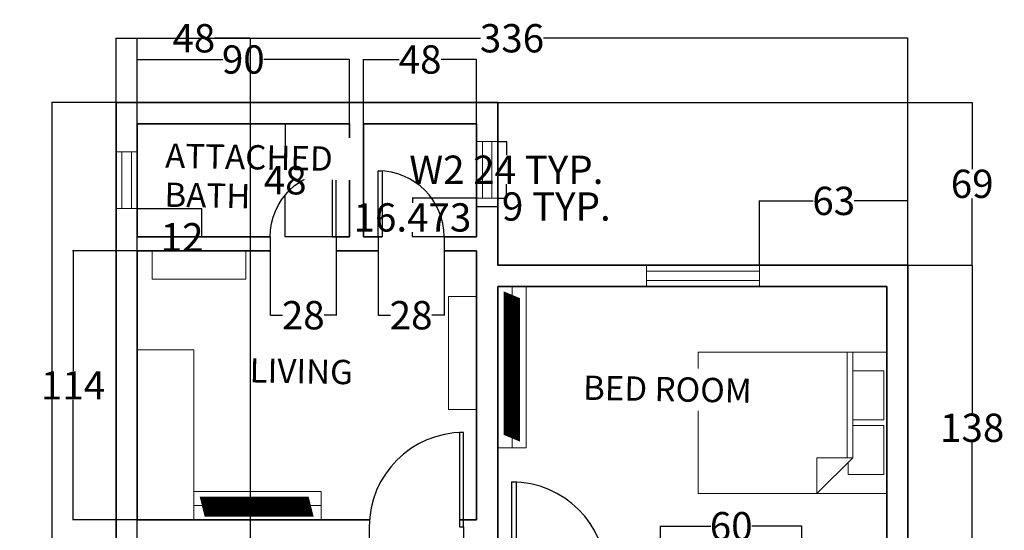
# Model space of a CAD drawing. Units: inches. Extents: x 424 to 1593, y 6 to 578.
# Tile 4 of 4: x 1175 to 1593, y 361 to 578. Entities that reach past the tile are written whole.
import ezdxf

# ---------------------------------------------------------------- set-up
doc = ezdxf.new("R2010")
doc.units = ezdxf.units.IN
doc.header["$MEASUREMENT"] = 0
for name, color, linetype, lineweight in [('A-ANNO-DIMS', 2, 'Continuous', 18), ('A-AREA-IDEN', 7, 'Continuous', 18), ('A-DOOR', 3, 'Continuous', 25), ('A-FLOR-CASE', 9, 'Continuous', 18), ('A-FLOR-CASE-PATT', 252, 'Continuous', 13), ('A-FURN', 8, 'Continuous', 18), ('A-GLAZ', 4, 'Continuous', 18), ('A-WALL', 7, 'Continuous', 35)]:
    doc.layers.add(name, color=color, linetype=linetype, lineweight=lineweight)
doc.styles.get("Standard").update_dxf_attribs({"font": 'arial.ttf'})
doc.dimstyles.get("Standard").update_dxf_attribs({"dimtxt": 12, "dimasz": 0.18, "dimexe": 0.18, "dimexo": 0.0625, "dimgap": 0.09, "dimtad": 0, "dimtih": 1, "dimtoh": 1, "dimdec": 0, "dimzin": 0, "dimdsep": 46, "dimlunit": 3, "dimtxsty": 'Standard', "dimcen": 0.09, "dimadec": 0, "dimazin": 0, "dimtfac": 1, "dimtdec": 0, "dimtofl": 0, "dimtmove": 0, "dimatfit": 3, "dimfxl": 1, "dimtolj": 1, "dimtzin": 0, "dimarcsym": 0})

# ---------------------------------------------------------------- blocks, each defined once
blk = doc.blocks.new('*U3')
for p, q in [((0, 0), (0, -6)), ((-40, 0), (-40, -6))]:
    blk.add_line(p, q)
blk.add_lwpolyline([(0, 0), (0, 40), (-1.75, 40), (-1.75, 0)], close=True)
blk.add_arc((0, 0), 40, 90, 180)
blk = doc.blocks.new('*U6')
for p, q in [((0, 0), (0, -6)), ((40, 0), (40, -6))]:
    blk.add_line(p, q)
blk.add_lwpolyline([(0, 0), (0, 40), (1.75, 40), (1.75, 0)], close=True)
blk.add_arc((0, 0), 40, 0, 90)
blk = doc.blocks.new('*U7')
for p, q in [((0, 0), (0, -6)), ((28, 0), (28, -6))]:
    blk.add_line(p, q)
blk.add_lwpolyline([(0, 0), (0, 28), (1.75, 28), (1.75, 0)], close=True)
blk.add_arc((0, 0), 28, 0, 90)
blk = doc.blocks.new('Bed - Queen')
for p, q in [((0, -80.00003), (0, 0)), ((0, 0), (59.99999, 0)), ((59.99999, 0), (59.99999, -80.00003)), ((7.99999, -1.2), (28.79998, -1.2)), ((7.99999, -14.4), (7.99999, -1.2)), ((28.79998, -1.2), (28.79998, -14.4)), ((31.19999, -1.2), (51.99999, -1.2)), ((31.19999, -14.4), (31.19999, -1.2)), ((51.99999, -1.2), (51.99999, -16.4)), ((0, -14.4), (44.8, -14.4)), ((59.99999, -29.6), (44.8, -14.4)), ((44.8, -14.4), (44.8, -29.6)), ((51.99999, -16.4), (46.79936, -16.4)), ((44.8, -16.8), (0, -16.8)), ((44.8, -29.6), (59.99999, -29.6)), ((59.99999, -80.00003), (0, -80.00003))]:
    blk.add_line(p, q)
blk = doc.blocks.new('WIN-48IN')
for p, q in [((2.5, 48), (2.5, 0)), ((6.5, 48), (6.5, 0))]:
    blk.add_line(p, q)
blk.add_lwpolyline([(0, 48), (9, 48), (9, 0), (0, 0)], close=True)
blk = doc.blocks.new('WIN-24IN')
for p, q in [((2.5, 0), (2.5, 24)), ((6.5, 0), (6.5, 24))]:
    blk.add_line(p, q)
blk.add_lwpolyline([(9, 0), (0, 0), (0, 24), (9, 24)], close=True)
blk = doc.blocks.new('CASEWORK-48X12')
blk.add_lwpolyline([(12, 48), (0, 48), (0, 0), (12, 0)], close=True)
blk = doc.blocks.new('*D14')
at = {"layer": 'A-ANNO-DIMS', "color": 0, "lineweight": -2, "transparency": 16777216}
for p, q in [((1377.79, 526), (1381.51, 526)), ((1381.33, 525.82), (1381.33, 520.12)), ((1381.33, 502.18), (1381.33, 507.88)), ((1377.79, 502), (1381.51, 502))]:
    blk.add_line(p, q, dxfattribs=at)
at = {"layer": 'A-ANNO-DIMS', "color": 0, "transparency": 16777216}
for points in [[(1381.3, 525.82), (1381.36, 525.82), (1381.33, 526)], [(1381.3, 502.18), (1381.36, 502.18), (1381.33, 502)]]:
    blk.add_solid(points, dxfattribs=at)
at = {"layer": 'Defpoints', "color": 0, "transparency": 16777216}
for p in [(1377.73, 526), (1381.33, 526), (1377.73, 502)]:
    blk.add_point(p, dxfattribs=at)
at = {"layer": 'A-ANNO-DIMS', "color": 0, "transparency": 16777216, "insert": (1381.33, 514), "char_height": 12, "attachment_point": 5}
blk.add_mtext('\\A1;W2 24 TYP.', dxfattribs=at)
blk = doc.blocks.new('*D15')
at = {"layer": 'A-ANNO-DIMS', "color": 0, "lineweight": -2, "transparency": 16777216}
for p, q in [((1368.73, 501.94), (1368.73, 498.22)), ((1377.73, 501.94), (1377.73, 498.22)), ((1368.91, 498.4), (1377.55, 498.4)), ((1377.73, 498.4), (1377.91, 498.4))]:
    blk.add_line(p, q, dxfattribs=at)
at = {"layer": 'A-ANNO-DIMS', "color": 0, "transparency": 16777216}
for points in [[(1368.91, 498.43), (1368.91, 498.37), (1368.73, 498.4)], [(1377.55, 498.43), (1377.55, 498.37), (1377.73, 498.4)]]:
    blk.add_solid(points, dxfattribs=at)
at = {"layer": 'Defpoints', "color": 0, "transparency": 16777216}
for p in [(1368.73, 502), (1377.73, 502), (1377.73, 498.4)]:
    blk.add_point(p, dxfattribs=at)
at = {"layer": 'A-ANNO-DIMS', "color": 0, "transparency": 16777216, "insert": (1402.54, 498.4), "char_height": 12, "attachment_point": 5}
blk.add_mtext('\\A1;9 TYP.', dxfattribs=at)
blk = doc.blocks.new('*D48')
at = {"layer": 'A-ANNO-DIMS', "color": 0, "lineweight": -2, "transparency": 16777216}
for p, q in [((1215.73, 542.59), (1215.73, 569.96)), ((1215.91, 569.78), (1370.39, 569.78)), ((1551.55, 569.78), (1397.07, 569.78)), ((1551.73, 473.59), (1551.73, 569.96))]:
    blk.add_line(p, q, dxfattribs=at)
at = {"layer": 'A-ANNO-DIMS', "color": 0, "transparency": 16777216}
for points in [[(1215.91, 569.81), (1215.91, 569.75), (1215.73, 569.78)], [(1551.55, 569.81), (1551.55, 569.75), (1551.73, 569.78)]]:
    blk.add_solid(points, dxfattribs=at)
at = {"layer": 'Defpoints', "color": 0, "transparency": 16777216}
for p in [(1551.73, 569.78), (1215.73, 542.53), (1551.73, 473.53)]:
    blk.add_point(p, dxfattribs=at)
at = {"layer": 'A-ANNO-DIMS', "color": 0, "transparency": 16777216, "insert": (1383.73, 569.78), "char_height": 12, "attachment_point": 5}
blk.add_mtext('\\A1;336', dxfattribs=at)
blk = doc.blocks.new('*D49')
at = {"layer": 'A-ANNO-DIMS', "color": 0, "lineweight": -2, "transparency": 16777216}
for p, q in [((1215.66, 542.53), (1188.3, 542.53)), ((1188.48, 542.35), (1188.48, 302.75)), ((1188.48, 50.71), (1188.48, 290.31)), ((1215.66, 50.53), (1188.3, 50.53))]:
    blk.add_line(p, q, dxfattribs=at)
at = {"layer": 'A-ANNO-DIMS', "color": 0, "transparency": 16777216}
for points in [[(1188.45, 542.35), (1188.51, 542.35), (1188.48, 542.53)], [(1188.45, 50.71), (1188.51, 50.71), (1188.48, 50.53)]]:
    blk.add_solid(points, dxfattribs=at)
at = {"layer": 'Defpoints', "color": 0, "transparency": 16777216}
for p in [(1188.48, 542.53), (1215.73, 542.53), (1215.73, 50.53)]:
    blk.add_point(p, dxfattribs=at)
at = {"layer": 'A-ANNO-DIMS', "color": 0, "transparency": 16777216, "insert": (1188.48, 296.53), "char_height": 12, "attachment_point": 5}
blk.add_mtext('\\A1;492', dxfattribs=at)
blk = doc.blocks.new('*D53')
at = {"layer": 'A-ANNO-DIMS', "color": 0, "lineweight": -2, "transparency": 16777216}
for p, q in [((1224.66, 479.53), (1197.3, 479.53)), ((1197.48, 479.35), (1197.48, 428.64)), ((1197.48, 365.71), (1197.48, 416.42)), ((1224.66, 365.53), (1197.3, 365.53))]:
    blk.add_line(p, q, dxfattribs=at)
at = {"layer": 'A-ANNO-DIMS', "color": 0, "transparency": 16777216}
for points in [[(1197.45, 479.35), (1197.51, 479.35), (1197.48, 479.53)], [(1197.45, 365.71), (1197.51, 365.71), (1197.48, 365.53)]]:
    blk.add_solid(points, dxfattribs=at)
at = {"layer": 'Defpoints', "color": 0, "transparency": 16777216}
for p in [(1197.48, 479.53), (1224.73, 479.53), (1224.73, 365.53)]:
    blk.add_point(p, dxfattribs=at)
at = {"layer": 'A-ANNO-DIMS', "color": 0, "transparency": 16777216, "insert": (1197.48, 422.53), "char_height": 12, "attachment_point": 5}
blk.add_mtext('\\A1;114', dxfattribs=at)
blk = doc.blocks.new('*D54')
at = {"layer": 'A-ANNO-DIMS', "color": 0, "lineweight": -2, "transparency": 16777216}
for p, q in [((1314.66, 533.53), (1287.3, 533.53)), ((1287.48, 533.35), (1287.48, 515.75)), ((1287.48, 485.71), (1287.48, 503.31)), ((1314.66, 485.53), (1287.3, 485.53))]:
    blk.add_line(p, q, dxfattribs=at)
at = {"layer": 'A-ANNO-DIMS', "color": 0, "transparency": 16777216}
for points in [[(1287.45, 533.35), (1287.51, 533.35), (1287.48, 533.53)], [(1287.45, 485.71), (1287.51, 485.71), (1287.48, 485.53)]]:
    blk.add_solid(points, dxfattribs=at)
at = {"layer": 'Defpoints', "color": 0, "transparency": 16777216}
for p in [(1287.48, 533.53), (1314.73, 533.53), (1314.73, 485.53)]:
    blk.add_point(p, dxfattribs=at)
at = {"layer": 'A-ANNO-DIMS', "color": 0, "transparency": 16777216, "insert": (1287.48, 509.53), "char_height": 12, "attachment_point": 5}
blk.add_mtext('\\A1;48', dxfattribs=at)
blk = doc.blocks.new('*D58')
at = {"layer": 'A-ANNO-DIMS', "color": 0, "lineweight": -2, "transparency": 16777216}
for p, q in [((1551.79, 473.53), (1579.16, 473.53)), ((1578.98, 473.35), (1578.98, 410.75)), ((1578.98, 335.71), (1578.98, 398.31)), ((1542.79, 335.53), (1579.16, 335.53))]:
    blk.add_line(p, q, dxfattribs=at)
at = {"layer": 'A-ANNO-DIMS', "color": 0, "transparency": 16777216}
for points in [[(1578.95, 473.35), (1579.01, 473.35), (1578.98, 473.53)], [(1578.95, 335.71), (1579.01, 335.71), (1578.98, 335.53)]]:
    blk.add_solid(points, dxfattribs=at)
at = {"layer": 'Defpoints', "color": 0, "transparency": 16777216}
for p in [(1551.73, 473.53), (1578.98, 473.53), (1542.73, 335.53)]:
    blk.add_point(p, dxfattribs=at)
at = {"layer": 'A-ANNO-DIMS', "color": 0, "transparency": 16777216, "insert": (1578.98, 404.53), "char_height": 12, "attachment_point": 5}
blk.add_mtext('\\A1;138', dxfattribs=at)
blk = doc.blocks.new('*D59')
at = {"layer": 'A-ANNO-DIMS', "color": 0, "lineweight": -2, "transparency": 16777216}
for p, q in [((1377.79, 542.53), (1579.16, 542.53)), ((1578.98, 542.35), (1578.98, 514.25)), ((1578.98, 473.71), (1578.98, 501.81)), ((1551.79, 473.53), (1579.16, 473.53))]:
    blk.add_line(p, q, dxfattribs=at)
at = {"layer": 'A-ANNO-DIMS', "color": 0, "transparency": 16777216}
for points in [[(1578.95, 542.35), (1579.01, 542.35), (1578.98, 542.53)], [(1578.95, 473.71), (1579.01, 473.71), (1578.98, 473.53)]]:
    blk.add_solid(points, dxfattribs=at)
at = {"layer": 'Defpoints', "color": 0, "transparency": 16777216}
for p in [(1377.73, 542.53), (1578.98, 542.53), (1551.73, 473.53)]:
    blk.add_point(p, dxfattribs=at)
at = {"layer": 'A-ANNO-DIMS', "color": 0, "transparency": 16777216, "insert": (1578.98, 508.03), "char_height": 12, "attachment_point": 5}
blk.add_mtext('\\A1;69', dxfattribs=at)
blk = doc.blocks.new('*D60')
at = {"layer": 'A-ANNO-DIMS', "color": 0, "lineweight": -2, "transparency": 16777216}
for p, q in [((1224.73, 533.59), (1224.73, 560.96)), ((1224.91, 560.78), (1261.06, 560.78)), ((1314.55, 560.78), (1278.39, 560.78)), ((1314.73, 533.59), (1314.73, 560.96))]:
    blk.add_line(p, q, dxfattribs=at)
at = {"layer": 'A-ANNO-DIMS', "color": 0, "transparency": 16777216}
for points in [[(1224.91, 560.81), (1224.91, 560.75), (1224.73, 560.78)], [(1314.55, 560.81), (1314.55, 560.75), (1314.73, 560.78)]]:
    blk.add_solid(points, dxfattribs=at)
at = {"layer": 'Defpoints', "color": 0, "transparency": 16777216}
for p in [(1314.73, 560.78), (1224.73, 533.53), (1314.73, 533.53)]:
    blk.add_point(p, dxfattribs=at)
at = {"layer": 'A-ANNO-DIMS', "color": 0, "transparency": 16777216, "insert": (1269.73, 560.78), "char_height": 12, "attachment_point": 5}
blk.add_mtext('\\A1;90', dxfattribs=at)
blk = doc.blocks.new('*D61')
at = {"layer": 'A-ANNO-DIMS', "color": 0, "lineweight": -2, "transparency": 16777216}
for p, q in [((1320.73, 533.59), (1320.73, 560.96)), ((1320.91, 560.78), (1335.79, 560.78)), ((1368.55, 560.78), (1353.67, 560.78)), ((1368.73, 533.59), (1368.73, 560.96))]:
    blk.add_line(p, q, dxfattribs=at)
at = {"layer": 'A-ANNO-DIMS', "color": 0, "transparency": 16777216}
for points in [[(1320.91, 560.81), (1320.91, 560.75), (1320.73, 560.78)], [(1368.55, 560.81), (1368.55, 560.75), (1368.73, 560.78)]]:
    blk.add_solid(points, dxfattribs=at)
at = {"layer": 'Defpoints', "color": 0, "transparency": 16777216}
for p in [(1368.73, 560.78), (1320.73, 533.53), (1368.73, 533.53)]:
    blk.add_point(p, dxfattribs=at)
at = {"layer": 'A-ANNO-DIMS', "color": 0, "transparency": 16777216, "insert": (1344.73, 560.78), "char_height": 12, "attachment_point": 5}
blk.add_mtext('\\A1;48', dxfattribs=at)
blk = doc.blocks.new('*D63')
at = {"layer": 'A-ANNO-DIMS', "color": 0, "lineweight": -2, "transparency": 16777216}
for p, q in [((1224.73, 59.59), (1224.73, 569.96)), ((1224.91, 569.78), (1239.79, 569.78)), ((1272.55, 569.78), (1257.67, 569.78)), ((1272.73, 59.59), (1272.73, 569.96))]:
    blk.add_line(p, q, dxfattribs=at)
at = {"layer": 'A-ANNO-DIMS', "color": 0, "transparency": 16777216}
for points in [[(1224.91, 569.81), (1224.91, 569.75), (1224.73, 569.78)], [(1272.55, 569.81), (1272.55, 569.75), (1272.73, 569.78)]]:
    blk.add_solid(points, dxfattribs=at)
at = {"layer": 'Defpoints', "color": 0, "transparency": 16777216}
for p in [(1272.73, 569.78), (1224.73, 59.53), (1272.73, 59.53)]:
    blk.add_point(p, dxfattribs=at)
at = {"layer": 'A-ANNO-DIMS', "color": 0, "transparency": 16777216, "insert": (1248.73, 569.78), "char_height": 12, "attachment_point": 5}
blk.add_mtext('\\A1;48', dxfattribs=at)
blk = doc.blocks.new('*D64')
at = {"layer": 'A-ANNO-DIMS', "color": 0, "lineweight": -2, "transparency": 16777216}
for p, q in [((1488.73, 473.59), (1488.73, 500.96)), ((1488.91, 500.78), (1511.51, 500.78)), ((1551.55, 500.78), (1528.95, 500.78)), ((1551.73, 473.59), (1551.73, 500.96))]:
    blk.add_line(p, q, dxfattribs=at)
at = {"layer": 'A-ANNO-DIMS', "color": 0, "transparency": 16777216}
for points in [[(1488.91, 500.81), (1488.91, 500.75), (1488.73, 500.78)], [(1551.55, 500.81), (1551.55, 500.75), (1551.73, 500.78)]]:
    blk.add_solid(points, dxfattribs=at)
at = {"layer": 'Defpoints', "color": 0, "transparency": 16777216}
for p in [(1551.73, 500.78), (1488.73, 473.53), (1551.73, 473.53)]:
    blk.add_point(p, dxfattribs=at)
at = {"layer": 'A-ANNO-DIMS', "color": 0, "transparency": 16777216, "insert": (1520.23, 500.78), "char_height": 12, "attachment_point": 5}
blk.add_mtext('\\A1;63', dxfattribs=at)
blk = doc.blocks.new('*D67')
at = {"layer": 'A-ANNO-DIMS', "color": 0, "lineweight": -2, "transparency": 16777216}
for p, q in [((1446.73, 335.59), (1446.73, 362.96)), ((1446.91, 362.78), (1468.03, 362.78)), ((1506.55, 362.78), (1485.42, 362.78)), ((1506.73, 335.59), (1506.73, 362.96))]:
    blk.add_line(p, q, dxfattribs=at)
at = {"layer": 'A-ANNO-DIMS', "color": 0, "transparency": 16777216}
for points in [[(1446.91, 362.81), (1446.91, 362.75), (1446.73, 362.78)], [(1506.55, 362.81), (1506.55, 362.75), (1506.73, 362.78)]]:
    blk.add_solid(points, dxfattribs=at)
at = {"layer": 'Defpoints', "color": 0, "transparency": 16777216}
for p in [(1506.73, 362.78), (1446.73, 335.53), (1506.73, 335.53)]:
    blk.add_point(p, dxfattribs=at)
at = {"layer": 'A-ANNO-DIMS', "color": 0, "transparency": 16777216, "insert": (1476.73, 362.78), "char_height": 12, "attachment_point": 5}
blk.add_mtext('\\A1;60', dxfattribs=at)
blk = doc.blocks.new('*D69')
at = {"layer": 'A-ANNO-DIMS', "color": 0, "lineweight": -2, "transparency": 16777216}
for p, q in [((1224.79, 497.53), (1252.16, 497.53)), ((1251.98, 497.35), (1251.98, 485.71)), ((1224.79, 485.53), (1252.16, 485.53)), ((1251.98, 485.35), (1251.8, 485.35)), ((1251.98, 485.53), (1251.98, 485.35))]:
    blk.add_line(p, q, dxfattribs=at)
at = {"layer": 'A-ANNO-DIMS', "color": 0, "transparency": 16777216}
for points in [[(1251.95, 497.35), (1252.01, 497.35), (1251.98, 497.53)], [(1251.95, 485.71), (1252.01, 485.71), (1251.98, 485.53)]]:
    blk.add_solid(points, dxfattribs=at)
at = {"layer": 'Defpoints', "color": 0, "transparency": 16777216}
for p in [(1224.73, 497.53), (1224.73, 485.53), (1251.98, 485.53)]:
    blk.add_point(p, dxfattribs=at)
at = {"layer": 'A-ANNO-DIMS', "color": 0, "transparency": 16777216, "insert": (1243.74, 485.35), "char_height": 12, "attachment_point": 5}
blk.add_mtext('\\A1;12', dxfattribs=at)
blk = doc.blocks.new('*D70')
at = {"layer": 'A-ANNO-DIMS', "color": 0, "lineweight": -2, "transparency": 16777216}
for p, q in [((1368.66, 502), (1341.3, 502)), ((1341.48, 501.82), (1341.48, 499.99)), ((1368.66, 485.53), (1341.3, 485.53)), ((1341.48, 485.71), (1341.48, 487.55))]:
    blk.add_line(p, q, dxfattribs=at)
at = {"layer": 'A-ANNO-DIMS', "color": 0, "transparency": 16777216}
for points in [[(1341.45, 501.82), (1341.51, 501.82), (1341.48, 502)], [(1341.45, 485.71), (1341.51, 485.71), (1341.48, 485.53)]]:
    blk.add_solid(points, dxfattribs=at)
at = {"layer": 'Defpoints', "color": 0, "transparency": 16777216}
for p in [(1341.48, 502), (1368.73, 502), (1368.73, 485.53)]:
    blk.add_point(p, dxfattribs=at)
at = {"layer": 'A-ANNO-DIMS', "color": 0, "transparency": 16777216, "insert": (1341.48, 493.77), "char_height": 12, "attachment_point": 5}
blk.add_mtext('\\A1;16.473', dxfattribs=at)
blk = doc.blocks.new('*D72')
at = {"layer": 'A-ANNO-DIMS', "color": 0, "lineweight": -2, "transparency": 16777216}
for p, q in [((1281.17, 479.47), (1281.17, 452.1)), ((1309.17, 479.47), (1309.17, 452.1)), ((1281.35, 452.28), (1286.37, 452.28)), ((1308.99, 452.28), (1303.97, 452.28))]:
    blk.add_line(p, q, dxfattribs=at)
at = {"layer": 'A-ANNO-DIMS', "color": 0, "transparency": 16777216}
for points in [[(1281.35, 452.31), (1281.35, 452.25), (1281.17, 452.28)], [(1308.99, 452.31), (1308.99, 452.25), (1309.17, 452.28)]]:
    blk.add_solid(points, dxfattribs=at)
at = {"layer": 'Defpoints', "color": 0, "transparency": 16777216}
for p in [(1281.17, 479.53), (1309.17, 479.53), (1281.17, 452.28)]:
    blk.add_point(p, dxfattribs=at)
at = {"layer": 'A-ANNO-DIMS', "color": 0, "transparency": 16777216, "insert": (1295.17, 452.28), "char_height": 12, "attachment_point": 5}
blk.add_mtext('\\A1;28', dxfattribs=at)
blk = doc.blocks.new('*D73')
at = {"layer": 'A-ANNO-DIMS', "color": 0, "lineweight": -2, "transparency": 16777216}
for p, q in [((1326.92, 479.47), (1326.92, 452.1)), ((1354.92, 479.47), (1354.92, 452.1)), ((1327.1, 452.28), (1332.12, 452.28)), ((1354.74, 452.28), (1349.71, 452.28))]:
    blk.add_line(p, q, dxfattribs=at)
at = {"layer": 'A-ANNO-DIMS', "color": 0, "transparency": 16777216}
for points in [[(1327.1, 452.31), (1327.1, 452.25), (1326.92, 452.28)], [(1354.74, 452.31), (1354.74, 452.25), (1354.92, 452.28)]]:
    blk.add_solid(points, dxfattribs=at)
at = {"layer": 'Defpoints', "color": 0, "transparency": 16777216}
for p in [(1326.92, 479.53), (1354.92, 479.53), (1326.92, 452.28)]:
    blk.add_point(p, dxfattribs=at)
at = {"layer": 'A-ANNO-DIMS', "color": 0, "transparency": 16777216, "insert": (1340.92, 452.28), "char_height": 12, "attachment_point": 5}
blk.add_mtext('\\A1;28', dxfattribs=at)

msp = doc.modelspace()

# ---------------------------------------------------------------- hatches: boundary and pattern name
at = {"layer": 'A-FLOR-CASE-PATT'}
h = msp.add_hatch(dxfattribs=at)
h.set_pattern_fill('ANSI31', color=256, scale=1.178482, angle=112.399, style=0)
h.paths.add_polyline_path([(1380.271, 401.5574), (1387.0743, 398.7254), (1387.0743, 459.5193), (1380.271, 462.3513)])
h = msp.add_hatch(dxfattribs=at)
h.set_pattern_fill('ANSI31', color=256, scale=0.876872, angle=59.407, style=0)
h.paths.add_polyline_path([(1251.353, 375.2477), (1253.4904, 366.927), (1299.4817, 366.927), (1297.3443, 375.2477)])

# ---------------------------------------------------------------- linework, layer by layer
at = {"layer": 'A-FLOR-CASE'}
for p, q in [((1383.7275, 396.0092), (1383.7275, 464.5296)), ((1248.7275, 371.5296), (1302.7275, 371.5296))]:
    msp.add_line(p, q, dxfattribs=at)
for points in [[(1231.0828, 479.5296), (1270.7906, 479.5296), (1270.7906, 467.5296), (1231.0828, 467.5296)], [(1377.7275, 464.5296), (1389.7275, 464.5296), (1389.7275, 396.0092), (1377.7275, 396.0092)], [(1224.7275, 365.5296), (1248.7275, 365.5296), (1248.7275, 437.5296), (1224.7275, 437.5296)], [(1248.7275, 365.5296), (1302.7275, 365.5296), (1302.7275, 377.5296), (1248.7275, 377.5296)]]:
    msp.add_lwpolyline(points, close=True, dxfattribs=at)
at = {"layer": 'A-WALL'}
for p, q in [((1377.7275, 473.5296), (1377.7275, 542.5296)), ((1224.7275, 533.5296), (1314.7275, 533.5296)), ((1224.7275, 485.5296), (1224.7275, 533.5296)), ((1314.7275, 485.5296), (1314.7275, 533.5296)), ((1320.7275, 485.5296), (1320.7275, 533.5296)), ((1320.7275, 533.5296), (1368.7275, 533.5296)), ((1368.7275, 485.5296), (1368.7275, 533.5296)), ((1224.7275, 485.5296), (1281.1668, 485.5296)), ((1307.4168, 485.5296), (1314.7275, 485.5296)), ((1320.7275, 485.5296), (1328.665, 485.5296)), ((1354.915, 485.5296), (1368.7275, 485.5296)), ((1224.7275, 479.5296), (1281.1668, 479.5296)), ((1224.7275, 365.5296), (1224.7275, 479.5296)), ((1309.1668, 479.5296), (1326.915, 479.5296)), ((1326.915, 479.5296), (1320.915, 479.5296)), ((1354.915, 479.5296), (1368.7275, 479.5296)), ((1368.7275, 464.5296), (1368.7275, 479.5296)), ((1377.7275, 473.5296), (1551.7275, 473.5296)), ((1368.7275, 464.5296), (1368.7275, 365.5296)), ((1377.7275, 464.5296), (1542.7275, 464.5296)), ((1377.7275, 464.5296), (1377.7275, 344.5296)), ((1542.7275, 464.5296), (1542.7275, 344.5296)), ((1224.7275, 365.5296), (1323.2714, 365.5296)), ((1361.4088, 365.5296), (1368.7275, 365.5296))]:
    msp.add_line(p, q, dxfattribs=at)
for points in [[(1377.7275, 50.5296), (1215.7275, 50.5296), (1215.7275, 542.5296), (1377.7275, 542.5296)], [(1377.7275, 50.5296), (1215.7275, 50.5296), (1215.7275, 542.5296), (1377.7275, 542.5296)], [(1224.7275, 485.5296), (1224.7275, 533.5296), (1314.7275, 533.5296)], [(1320.7275, 533.5296), (1368.7275, 533.5296)], [(1224.7275, 365.5296), (1224.7275, 479.5296)], [(1551.7275, 473.5296), (1551.7275, 110.5296)], [(1542.7275, 464.5296), (1542.7275, 344.5296)]]:
    msp.add_lwpolyline(points, dxfattribs=at)

# ---------------------------------------------------------------- block references
at = {"layer": 'A-DOOR', "xscale": -1}
msp.add_blockref('*U7', (1309.1668, 485.5296), dxfattribs=at)
at = {"layer": 'A-DOOR'}
for name, p in [('*U7', (1326.915, 485.5296)), ('*U3', (1363.1588, 362.5296)), ('*U6', (1383.7159, 341.5296))]:
    msp.add_blockref(name, p, dxfattribs=at)
at = {"layer": 'A-FLOR-CASE'}
msp.add_blockref('CASEWORK-48X12', (1356.7276, 412.266), dxfattribs=at)
at = {"layer": 'A-FURN', "rotation": 270}
msp.add_blockref('Bed - Queen', (1542.7275, 436.6366), dxfattribs=at)
at = {"layer": 'A-GLAZ'}
for p in [(1368.727, 502.003), (1215.727, 497.5297)]:
    msp.add_blockref('WIN-24IN', p, dxfattribs=at)
at = {"layer": 'A-GLAZ', "rotation": 89.99999999999996}
msp.add_blockref('WIN-48IN', (1488.7276, 464.5297), dxfattribs=at)

# ---------------------------------------------------------------- texts
at = {"layer": 'A-AREA-IDEN'}
for s, p in [('BATH', (1236.1855, 498.3095)), ('LIVING', (1272.3204, 423.7817))]:
    msp.add_text(s, height=10.30671, rotation=358.915866, dxfattribs=at).set_placement(p)

# ---------------------------------------------------------------- dimensions: what is measured, and where the dimension line sits
at = {"layer": 'A-ANNO-DIMS'}
for base, p1, p2, picture, middle in [((1314.7275, 560.7796), (1224.7275, 533.5296), (1314.7275, 533.5296), '*D60', (1269.7275, 560.7796)), ((1368.7275, 560.7796), (1320.7275, 533.5296), (1368.7275, 533.5296), '*D61', (1344.7275, 560.7796)), ((1506.7275, 362.7796), (1446.7275, 335.5296), (1506.7275, 335.5296), '*D67', (1476.7275, 362.7796))]:
    dim = msp.add_linear_dim(base=base, p1=p1, p2=p2, dimstyle='Standard', override={"dimdec": 0, "dimlfac": 1, "dimrnd": 0, "dimzin": 0, "dimdsep": 46, "dimlunit": 2}, dxfattribs=at)
    dim.commit()
    dim.dimension.update_dxf_attribs({"geometry": picture, "text_midpoint": middle})
for base, p1, p2, angle, override, picture, middle in [((1188.4775, 542.5296), (1215.7275, 50.5296), (1215.7275, 542.5296), 90, {"dimdec": 0, "dimlfac": 1, "dimrnd": 0, "dimzin": 0, "dimdsep": 46, "dimlunit": 2}, '*D49', (1188.4775, 296.5296)), ((1578.9775, 542.5296), (1551.7275, 473.5296), (1377.7275, 542.5296), 90, {"dimdec": 0, "dimlfac": 1, "dimrnd": 0, "dimzin": 0, "dimdsep": 46, "dimlunit": 2}, '*D59', (1578.9775, 508.0296)), ((1551.7275, 500.7796), (1488.7275, 473.5296), (1551.7275, 473.5296), 0, {"dimdec": 0, "dimlfac": 1, "dimrnd": 0, "dimzin": 0, "dimdsep": 46, "dimlunit": 2}, '*D64', (1520.2275, 500.7796)), ((1341.4775, 502.0029), (1368.7275, 485.5296), (1368.7275, 502.0029), 90, {"dimdec": 3, "dimlfac": 1, "dimrnd": 0, "dimzin": 0, "dimdsep": 46, "dimlunit": 2}, '*D70', (1341.4775, 493.7663)), ((1251.9775, 485.5296), (1224.7275, 497.5296), (1224.7275, 485.5296), 270, {"dimdec": 0, "dimlfac": 1, "dimrnd": 0, "dimzin": 0, "dimdsep": 46, "dimlunit": 2}, '*D69', (1243.7389, 485.3496)), ((1197.4775, 479.5296), (1224.7275, 365.5296), (1224.7275, 479.5296), 90, {"dimdec": 0, "dimlfac": 1, "dimrnd": 0, "dimzin": 0, "dimdsep": 46, "dimlunit": 2}, '*D53', (1197.4775, 422.5296)), ((1281.1668, 452.2796), (1309.1668, 479.5296), (1281.1668, 479.5296), 180, {"dimdec": 0, "dimlfac": 1, "dimrnd": 0, "dimzin": 0, "dimdsep": 46, "dimlunit": 2}, '*D72', (1295.1668, 452.2796)), ((1326.915, 452.2796), (1354.915, 479.5296), (1326.915, 479.5296), 180, {"dimdec": 0, "dimlfac": 1, "dimrnd": 0, "dimzin": 0, "dimdsep": 46, "dimlunit": 2}, '*D73', (1340.915, 452.2796)), ((1578.9775, 473.5296), (1542.7275, 335.5296), (1551.7275, 473.5296), 90, {"dimdec": 0, "dimlfac": 1, "dimrnd": 0, "dimzin": 0, "dimdsep": 46, "dimlunit": 2}, '*D58', (1578.9775, 404.5296))]:
    dim = msp.add_linear_dim(base=base, p1=p1, p2=p2, angle=angle, dimstyle='Standard', override=override, dxfattribs=at)
    dim.commit()
    dim.dimension.update_dxf_attribs({"geometry": picture, "text_midpoint": middle})
dim = msp.add_linear_dim(base=(1381.3275, 526.0029), p1=(1377.7275, 502.0029), p2=(1377.7275, 526.0029), angle=90, text='W2 <> TYP.', dimstyle='Standard', override={"dimdec": 0, "dimlfac": 1, "dimrnd": 0, "dimzin": 0, "dimdsep": 46, "dimlunit": 2}, dxfattribs=at)
dim.commit()
dim.dimension.update_dxf_attribs({"geometry": '*D14', "text_midpoint": (1381.3275, 514.0029)})
dim = msp.add_linear_dim(base=(1377.7275, 498.4029), p1=(1368.7275, 502.0029), p2=(1377.7275, 502.0029), text='<> TYP.', dimstyle='Standard', override={"dimdec": 0, "dimlfac": 1, "dimrnd": 0, "dimzin": 0, "dimdsep": 46, "dimlunit": 2}, dxfattribs=at)
dim.commit()
dim.dimension.update_dxf_attribs({"geometry": '*D15', "text_midpoint": (1402.5418, 498.4029)})

# ---------------------------------------------------------------- next in the draw order: wipeouts: each hides what was drawn before it
for points in [[(1232.7994, 511.1495), (1316.8494, 509.559), (1317.1876, 527.4287), (1233.1375, 529.0193)], [(1411.1729, 412.6964), (1494.6255, 411.1172), (1494.9638, 428.9939), (1411.5112, 430.5732)]]:
    msp.add_wipeout(points).dxf.layer = 'A-AREA-IDEN'

# ---------------------------------------------------------------- next in the draw order: texts
at = {"layer": 'A-AREA-IDEN'}
for s, p in [('ATTACHED', (1236.4987, 514.8633)), ('BED ROOM', (1413.7968, 416.4306))]:
    msp.add_text(s, height=10.30671, rotation=358.915866, dxfattribs=at).set_placement(p)

# ---------------------------------------------------------------- next in the draw order: dimensions: what is measured, and where the dimension line sits
at = {"layer": 'A-ANNO-DIMS'}
for base, p1, p2, picture, middle in [((1551.7275, 569.7796), (1215.7275, 542.5296), (1551.7275, 473.5296), '*D48', (1383.7275, 569.7796)), ((1272.7275, 569.7796), (1224.7275, 59.5296), (1272.7275, 59.5296), '*D63', (1248.7275, 569.7796))]:
    dim = msp.add_linear_dim(base=base, p1=p1, p2=p2, dimstyle='Standard', override={"dimdec": 0, "dimlfac": 1, "dimrnd": 0, "dimzin": 0, "dimdsep": 46, "dimlunit": 2}, dxfattribs=at)
    dim.commit()
    dim.dimension.update_dxf_attribs({"geometry": picture, "text_midpoint": middle})
dim = msp.add_linear_dim(base=(1287.4775, 533.5296), p1=(1314.7275, 485.5296), p2=(1314.7275, 533.5296), angle=90, dimstyle='Standard', override={"dimdec": 0, "dimlfac": 1, "dimrnd": 0, "dimzin": 0, "dimdsep": 46, "dimlunit": 2}, dxfattribs=at)
dim.commit()
dim.dimension.update_dxf_attribs({"geometry": '*D54', "text_midpoint": (1287.4775, 509.5296)})

doc.saveas('drawing.dxf')
